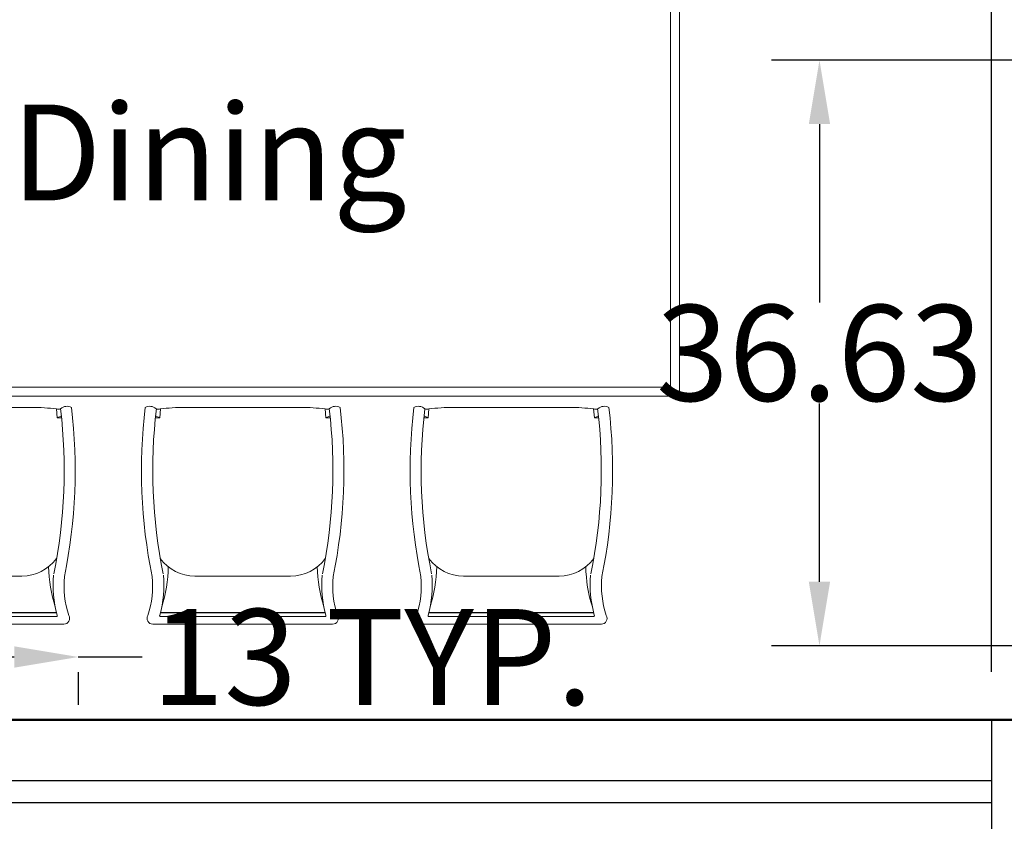
# Model space of a CAD drawing. Units: inches. Extents: x 89 to 490, y -59 to 378.
# Tile 12 of 20: x 339 to 400, y 7 to 58. Entities that reach past the tile are written whole.
import ezdxf

# ---------------------------------------------------------------- set-up
doc = ezdxf.new("R2010")
doc.units = ezdxf.units.IN
doc.header["$MEASUREMENT"] = 0
for name, color, linetype, lineweight in [('A-ANNO-DIMS', 2, 'Continuous', 18), ('A-AREA-IDEN', 7, 'Continuous', 18), ('Dining Table', 155, 'Continuous', 18), ('Outer Walls', 12, 'Continuous', 50), ('Windows', 171, 'Continuous', 25)]:
    doc.layers.add(name, color=color, linetype=linetype, lineweight=lineweight)
doc.styles.get("Standard").update_dxf_attribs({"font": 'arial.ttf'})
doc.dimstyles.get("Standard").update_dxf_attribs({"dimtxt": 6, "dimasz": 4, "dimexe": 3, "dimexo": 3, "dimgap": 0.09, "dimtad": 0, "dimtih": 1, "dimtoh": 1, "dimdec": 1, "dimzin": 0, "dimdsep": 46, "dimlunit": 3, "dimtxsty": 'Standard', "dimcen": 0.09, "dimadec": 0, "dimazin": 0, "dimtfac": 1, "dimtdec": 1, "dimtofl": 0, "dimtmove": 0, "dimatfit": 3, "dimfxl": 1, "dimtolj": 1, "dimtzin": 0, "dimarcsym": 0})

# ---------------------------------------------------------------- blocks, each defined once
blk = doc.blocks.new('Window')
for p, q in [((516.369, 95.253), (588.369, 95.253)), ((588.369, 93.853), (516.369, 93.853))]:
    blk.add_line(p, q)
blk.add_lwpolyline([(588.369, 99.053), (588.369, 90.053), (516.369, 90.053), (516.369, 99.053)], close=True)
blk = doc.blocks.new('A$C51F1')
at = {"color": 0}
for p, q in [((0.2273, 0.4758), (0.0436, 0.4758)), ((0.2273, 0.4676), (0.0439, 0.4676)), ((0.2273, 0.4668), (0.0439, 0.4668)), ((0.2273, 0.4758), (0.4111, 0.4758)), ((0.2273, 0.4676), (0.4107, 0.4676)), ((0.2273, 0.4668), (0.4107, 0.4668)), ((0.2273, 0.3858), (0.1205, 0.3858)), ((0.2273, 0.3858), (0.3341, 0.3858)), ((0.0417, 0.0321), (0.0321, 0.0321)), ((0.0417, 0.0321), (0.0326, 0.0278)), ((0.0435, 0.0127), (0.0417, 0.0321)), ((0.4112, 0.0127), (0.4129, 0.0321)), ((0.4129, 0.0321), (0.4225, 0.0321)), ((0.4129, 0.0321), (0.4221, 0.0278))]:
    blk.add_line(p, q, dxfattribs=at)
blk.add_lwpolyline([(0.4387, 0.4737, 0.102523), (0.4291, 0.3863, -0.080461), (0.4447, 0.0091, -0.3023), (0.4203, 0.012, 0.197932), (0.4111, 0.0127, -0.028193), (0.3571, 0.0091), (0.227, 0.0091), (0.097, 0.0091, -0.028193), (0.0429, 0.0127, 0.197932), (0.0338, 0.012, -0.3023), (0.0093, 0.0091, -0.080461), (0.0249, 0.3863, 0.102523), (0.0153, 0.4737, -0.587111), (0.0261, 0.4929), (0.4279, 0.4929, -0.587111)], format="xyb", close=True, dxfattribs=at)
for centre, radius, start, end in [((0.044, 0.4735), 0.00242, 100.345, 201.3742), ((-0.1898, 0.4063), 0.2409, 354.5513, 15.9626), ((0.0439, 0.4669), 0.000725, 87.3762, 197.5208), ((0.0438, 0.4664), 0.000433, 71.7715, 189.2202), ((0.6445, 0.4063), 0.2409, 164.0374, 185.4487), ((0.4107, 0.4669), 0.000725, 342.4792, 92.6238), ((0.4109, 0.4664), 0.000433, 350.7798, 108.2285), ((0.4106, 0.4735), 0.00242, 338.6258, 79.655), ((-0.2563, 0.3584), 0.3173, 1.1591, 17.5641), ((0.7109, 0.3584), 0.3173, 162.4359, 178.8409), ((1.1806, 0.1494), 1.1544, 168.4357, 186.8363), ((0.1214, 0.2879), 0.0978, 90.5164, 143.1927), ((0.3332, 0.2879), 0.0978, 36.8073, 89.4836), ((-0.7259, 0.1494), 1.1544, 353.1637, 11.5643), ((0.0397, 0.0013), 0.012, 71.7536, 116.5375), ((0.4149, 0.0013), 0.012, 63.4625, 108.2464)]:
    blk.add_arc(centre, radius, start, end, dxfattribs=at)
blk = doc.blocks.new('*D29')
at = {"layer": 'A-ANNO-DIMS', "color": 0, "lineweight": -2, "transparency": 16777216}
for p, q in [((333.431, 17.668), (338.483, 17.668)), ((342.483, 17.668), (346.483, 17.668)), ((329.431, 16.72), (329.431, 14.668)), ((342.483, 16.72), (342.483, 14.668))]:
    blk.add_line(p, q, dxfattribs=at)
at = {"layer": 'A-ANNO-DIMS', "color": 0, "transparency": 16777216}
for points in [[(333.431, 18.335), (333.431, 17.001), (329.431, 17.668)], [(338.483, 18.335), (338.483, 17.001), (342.483, 17.668)]]:
    blk.add_solid(points, dxfattribs=at)
at = {"layer": 'Defpoints', "color": 0, "transparency": 16777216}
for p in [(329.431, 19.72), (342.483, 19.72), (342.483, 17.668)]:
    blk.add_point(p, dxfattribs=at)
at = {"layer": 'A-ANNO-DIMS', "color": 0, "transparency": 16777216, "insert": (360.893, 17.668), "char_height": 6, "attachment_point": 5}
blk.add_mtext('\\A1;13 TYP.', dxfattribs=at)
blk = doc.blocks.new('*D37')
at = {"layer": 'A-ANNO-DIMS', "color": 0, "lineweight": -2, "transparency": 16777216}
for p, q in [((410.454, 13.741), (410.454, 17.741)), ((410.454, 17.741), (414.454, 17.741)), ((402.654, 13.741), (413.454, 13.741)), ((410.454, 8.741), (410.454, 9.741)), ((402.654, 4.741), (413.454, 4.741))]:
    blk.add_line(p, q, dxfattribs=at)
at = {"layer": 'A-ANNO-DIMS', "color": 0, "transparency": 16777216}
for points in [[(409.787, 9.741), (411.121, 9.741), (410.454, 13.741)], [(409.787, 8.741), (411.121, 8.741), (410.454, 4.741)]]:
    blk.add_solid(points, dxfattribs=at)
at = {"layer": 'Defpoints', "color": 0, "transparency": 16777216}
for p in [(399.654, 13.741), (410.454, 13.741), (399.654, 4.741)]:
    blk.add_point(p, dxfattribs=at)
at = {"layer": 'A-ANNO-DIMS', "color": 0, "transparency": 16777216, "insert": (416.517, 17.741), "char_height": 6, "attachment_point": 5}
blk.add_mtext('\\A1;9', dxfattribs=at)
blk = doc.blocks.new('*D48')
at = {"layer": 'A-ANNO-DIMS', "color": 0, "lineweight": -2, "transparency": 16777216}
for p, q in [((127.441, 10.741), (127.441, -49.809)), ((459.441, -29.659), (459.441, -49.809)), ((131.441, -46.809), (286.756, -46.809)), ((455.441, -46.809), (300.127, -46.809))]:
    blk.add_line(p, q, dxfattribs=at)
at = {"layer": 'A-ANNO-DIMS', "color": 0, "transparency": 16777216}
for points in [[(131.441, -46.143), (131.441, -47.476), (127.441, -46.809)], [(455.441, -46.143), (455.441, -47.476), (459.441, -46.809)]]:
    blk.add_solid(points, dxfattribs=at)
at = {"layer": 'Defpoints', "color": 0, "transparency": 16777216}
for p in [(127.441, 13.741), (459.441, -26.659), (459.441, -46.809)]:
    blk.add_point(p, dxfattribs=at)
at = {"layer": 'A-ANNO-DIMS', "color": 0, "transparency": 16777216, "insert": (293.441, -46.809), "char_height": 6, "attachment_point": 5}
blk.add_mtext('\\A1;332', dxfattribs=at)
blk = doc.blocks.new('*D64')
at = {"layer": 'A-ANNO-DIMS', "color": 0, "lineweight": -2, "transparency": 16777216}
for p, q in [((399.654, 16.741), (399.654, 376.891)), ((450.441, 16.741), (450.441, 376.891)), ((403.654, 373.891), (414.828, 373.891)), ((446.441, 373.891), (435.267, 373.891))]:
    blk.add_line(p, q, dxfattribs=at)
at = {"layer": 'A-ANNO-DIMS', "color": 0, "transparency": 16777216}
for points in [[(403.654, 374.558), (403.654, 373.225), (399.654, 373.891)], [(446.441, 374.558), (446.441, 373.225), (450.441, 373.891)]]:
    blk.add_solid(points, dxfattribs=at)
at = {"layer": 'Defpoints', "color": 0, "transparency": 16777216}
for p in [(450.441, 373.891), (399.654, 13.741), (450.441, 13.741)]:
    blk.add_point(p, dxfattribs=at)
at = {"layer": 'A-ANNO-DIMS', "color": 0, "transparency": 16777216, "insert": (425.048, 373.891), "char_height": 6, "attachment_point": 5}
blk.add_mtext('\\A1;50.79', dxfattribs=at)
blk = doc.blocks.new('*D72')
at = {"layer": 'A-ANNO-DIMS', "color": 0, "lineweight": -2, "transparency": 16777216}
for p, q in [((406.039, 55.006), (385.889, 55.006)), ((388.889, 51.006), (388.889, 39.845)), ((388.889, 22.374), (388.889, 33.534)), ((406.039, 18.374), (385.889, 18.374))]:
    blk.add_line(p, q, dxfattribs=at)
at = {"layer": 'A-ANNO-DIMS', "color": 0, "transparency": 16777216}
for points in [[(388.222, 51.006), (389.555, 51.006), (388.889, 55.006)], [(388.222, 22.374), (389.555, 22.374), (388.889, 18.374)]]:
    blk.add_solid(points, dxfattribs=at)
at = {"layer": 'Defpoints', "color": 0, "transparency": 16777216}
for p in [(388.889, 55.006), (409.039, 55.006), (409.039, 18.374)]:
    blk.add_point(p, dxfattribs=at)
at = {"layer": 'A-ANNO-DIMS', "color": 0, "transparency": 16777216, "insert": (388.889, 36.69), "char_height": 6, "attachment_point": 5}
blk.add_mtext('\\A1;36.63', dxfattribs=at)

msp = doc.modelspace()

# ---------------------------------------------------------------- linework, layer by layer
at = {"layer": 'Dining Table', "ltscale": 0.5}
for points in [[(324.0409, 33.9856), (380.116, 33.9856), (380.116, 62.0232), (324.0409, 62.0232)], [(324.6016, 34.5464), (379.5552, 34.5464), (379.5552, 61.4624), (324.6016, 61.4624)]]:
    msp.add_lwpolyline(points, close=True, dxfattribs=at)
at = {"layer": 'Outer Walls'}
msp.add_line((270.4414, 13.7413), (450.4414, 13.7413), dxfattribs=at)

# ---------------------------------------------------------------- block references
at = {"layer": 'Dining Table', "ltscale": 0.5, "yscale": 28.0375393373698, "zscale": 28.0375393373698, "rotation": 180}
for p, xscale in [((329.592, 33.5401), -28.0375393373698), ((346.4145, 33.5401), -28.0375393373698), ((375.9667, 33.5401), 28.0375393373698)]:
    msp.add_blockref('A$C51F1', p, dxfattribs=dict(at, xscale=xscale))
at = {"layer": 'Windows'}
msp.add_blockref('Window', (-188.7147, -85.3119), dxfattribs=at)

# ---------------------------------------------------------------- texts
at = {"layer": 'A-AREA-IDEN', "insert": (327.4748, 52.2324), "char_height": 6, "attachment_point": 1}
msp.add_mtext_dynamic_manual_height_columns('\\pxqc;Dining', width=46.403971, gutter_width=1, heights=[0], dxfattribs=at)

# ---------------------------------------------------------------- dimensions: what is measured, and where the dimension line sits
at = {"layer": 'A-ANNO-DIMS'}
for base, p1, p2, override, picture, middle in [((450.4414, 373.8913), (399.6539, 13.7413), (450.4414, 13.7413), {"dimdec": 2, "dimlfac": 1, "dimrnd": 0, "dimzin": 0, "dimdsep": 46, "dimlunit": 2}, '*D64', (425.0477, 373.8913)), ((459.4414, -46.8094), (127.4414, 13.7413), (459.4414, -26.6594), {"dimdec": 0, "dimlfac": 1, "dimrnd": 0, "dimzin": 0, "dimdsep": 46, "dimlunit": 2}, '*D48', (293.4414, -46.8094))]:
    dim = msp.add_linear_dim(base=base, p1=p1, p2=p2, dimstyle='Standard', override=override, dxfattribs=at)
    dim.commit()
    dim.dimension.update_dxf_attribs({"geometry": picture, "text_midpoint": middle})
for base, p1, p2, override, picture, middle in [((388.8888, 55.0057), (409.0388, 18.3742), (409.0388, 55.0057), {"dimdec": 2, "dimlfac": 1, "dimrnd": 0, "dimzin": 0, "dimdsep": 46, "dimlunit": 2}, '*D72', (388.8888, 36.69)), ((410.4539, 13.7413), (399.6539, 4.7413), (399.6539, 13.7413), {"dimdec": 0, "dimlfac": 1, "dimrnd": 0, "dimzin": 0, "dimdsep": 46, "dimlunit": 2}, '*D37', (416.5166, 17.7413))]:
    dim = msp.add_linear_dim(base=base, p1=p1, p2=p2, angle=90, dimstyle='Standard', override=override, dxfattribs=at)
    dim.commit()
    dim.dimension.update_dxf_attribs({"geometry": picture, "text_midpoint": middle})
dim = msp.add_linear_dim(base=(342.4828, 17.668), p1=(329.4308, 19.7198), p2=(342.4828, 19.7198), text='<> TYP.', dimstyle='Standard', override={"dimdec": 0, "dimlfac": 1, "dimrnd": 0, "dimzin": 0, "dimdsep": 46, "dimlunit": 2}, dxfattribs=at)
dim.commit()
dim.dimension.update_dxf_attribs({"geometry": '*D29', "text_midpoint": (360.8934, 17.668)})

doc.saveas('drawing.dxf')
